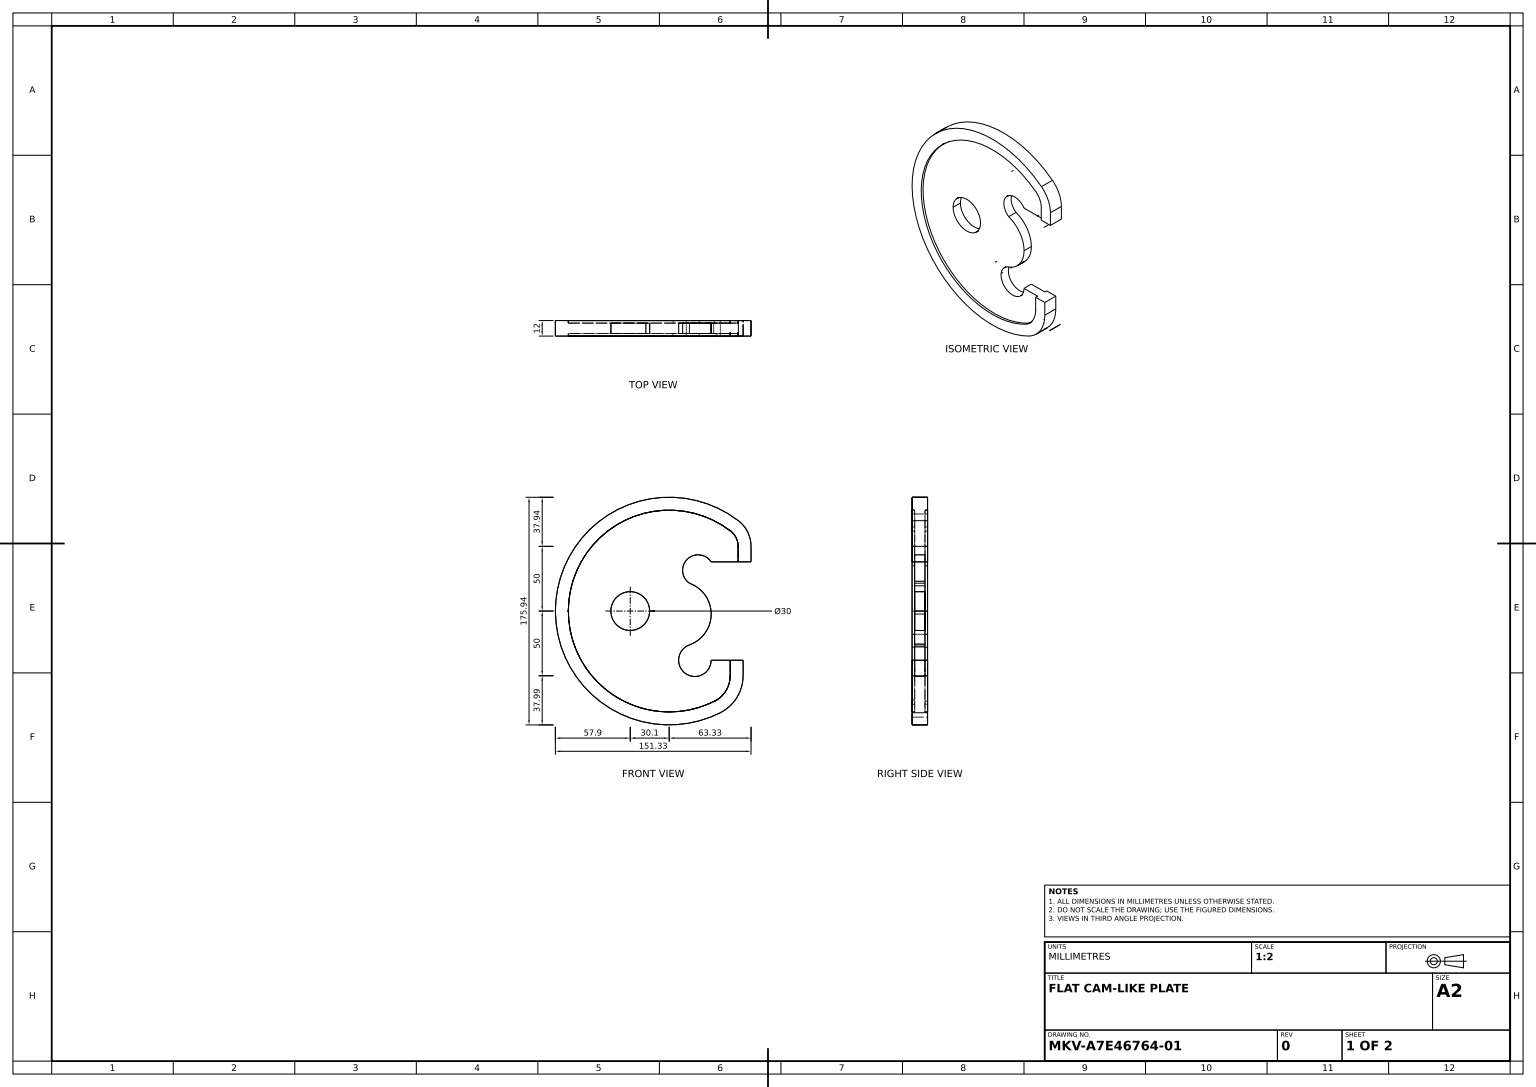
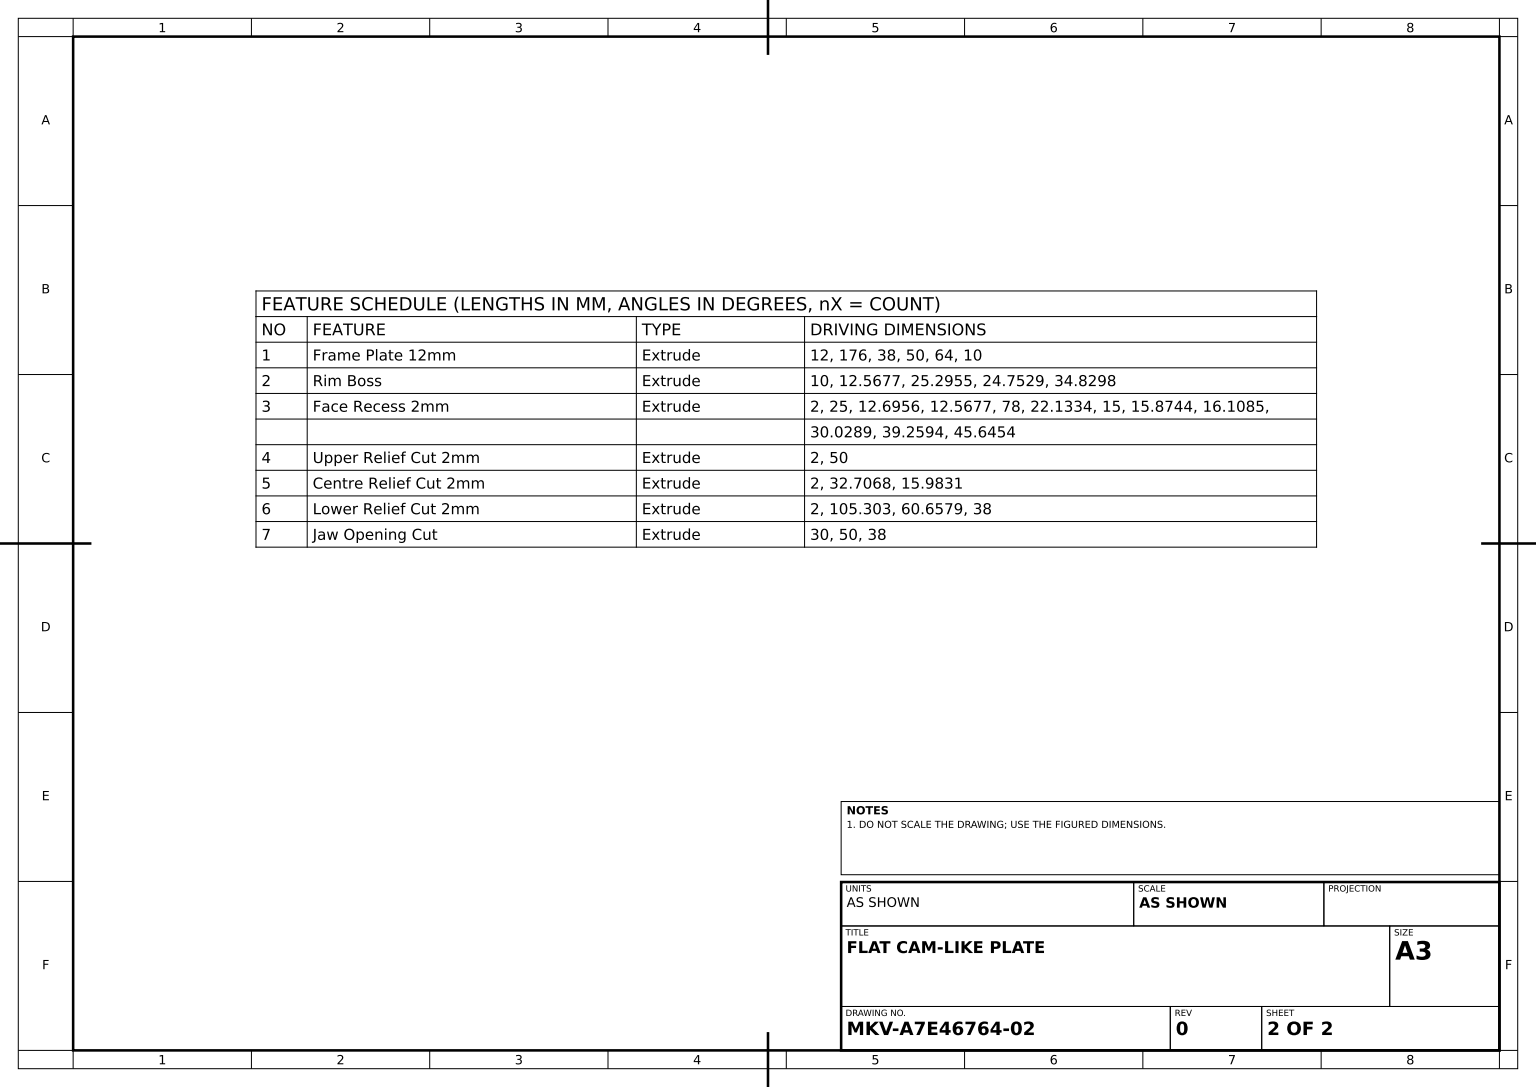
from build123d import *

# Parameters (mm, degrees)
FRAME_PLATE_12MM_DEPTH      = 6
RIM_BOSS_DEPTH              = 10
FACE_RECESS_2MM_DEPTH       = 2
UPPER_START                 = 2
UPPER_RELIEF_CUT_SKETCH_R   = 25
UPPER_RELIEF_CUT_2MM_DEPTH  = 2
CENTRE_RELIEF_CUT_2MM_DEPTH = 2
LOWER_RELIEF_CUT_SKETCH_R   = 52.651518039
LOWER_RELIEF_CUT_2MM_DEPTH  = 2
JAW_OPENING_SKETCH_R        = 15
JAW_OPENING_CUT_DEPTH       = 125.85191228


with BuildPart() as part:
    # Frame Profile Sketch → Frame Plate 12mm (new, symmetric)
    with BuildSketch(Plane.XY):
        with BuildLine():
            Line((57.219040426, -50), (57.219040426, -38))
            Line((57.219040426, -38), (47.219040426, -38))
            Line((47.219040426, -38), (47.219040426, -50))
            ThreePointArc((47.219040426, -50), (43.953561552, -61.533330749), (35.126520593, -69.642857143))
            ThreePointArc((35.126520593, -69.642857143), (-77.659797107, 7.277081367), (47.453139554, 61.904761905))
            ThreePointArc((47.453139554, 61.904761905), (51.779005163, 56.637617931), (53.327535793, 50))
            Line((53.327535793, 50), (53.327535793, 38))
            Line((53.327535793, 38), (63.327535793, 38))
            Line((63.327535793, 38), (63.327535793, 50))
            ThreePointArc((63.327535793, 50), (60.74665141, 61.062696552), (53.536875394, 69.841269841))
            ThreePointArc((53.536875394, 69.841269841), (-87.616181352, 8.210040517), (39.629920669, -78.571428571))
            ThreePointArc((39.629920669, -78.571428571), (52.469252974, -66.775753816), (57.219040426, -50))
        make_face()
    extrude(amount=FRAME_PLATE_12MM_DEPTH, both=True)

    # Rim Boss Sketch → Rim Boss (add)
    with BuildSketch(Plane.XY.offset(6)):
        with BuildLine():
            Line((53.327535793, 38), (32.46615526, 38))
            ThreePointArc((32.46615526, 38), (13.979168764, 40.044097465), (15.696546582, 21.523902608))
            ThreePointArc((15.696546582, 21.523902608), (32.534616457, -2.315840538), (15.696546582, -26.155583684))
            ThreePointArc((15.696546582, -26.155583684), (12.648035491, -48.265354025), (32.46615526, -38))
            Line((32.46615526, -38), (47.219040426, -38))
            Line((47.219040426, -38), (47.219040426, -50))
            ThreePointArc((47.219040426, -50), (43.953561552, -61.533330749), (35.126520593, -69.642857143))
            ThreePointArc((35.126520593, -69.642857143), (-77.659797107, 7.277081367), (47.453139554, 61.904761905))
            ThreePointArc((47.453139554, 61.904761905), (51.779005163, 56.637617931), (53.327535793, 50))
            Line((53.327535793, 50), (53.327535793, 38))
        make_face()
    extrude(amount=-RIM_BOSS_DEPTH)

    # Face Recess Sketch → Face Recess 2mm (cut)
    with BuildSketch(Plane.XY.offset(6)):
        with BuildLine():
            ThreePointArc((36.866729899, -68.73750233), (44.45885626, -60.703554629), (47.219040426, -50))
            Line((47.219040426, -50), (47.219040426, -38))
            Line((47.219040426, -38), (32.46615526, -38))
            ThreePointArc((32.46615526, -38), (30.153940112, -45.264433679), (24.06810264, -49.855829743))
            ThreePointArc((24.06810264, -49.855829743), (7.879587743, -42.091412935), (15.644004551, -25.902898038))
            ThreePointArc((15.644004551, -25.902898038), (32.325529371, -3.417209672), (17.682148152, 20.445959399))
            ThreePointArc((17.682148152, 20.445959399), (16.663921846, 20.938096482), (15.696546582, 21.523902608))
            ThreePointArc((15.696546582, 21.523902608), (13.979168764, 40.044097465), (32.46615526, 38))
            Line((32.46615526, 38), (53.327535793, 38))
            Line((53.327535793, 38), (53.327535793, 50))
            ThreePointArc((53.327535793, 50), (51.779005163, 56.637617931), (47.453139554, 61.904761905))
            ThreePointArc((47.453139554, 61.904761905), (-77.745163176, 6.299968474), (36.866729899, -68.73750233))
        make_face()
    extrude(amount=-FACE_RECESS_2MM_DEPTH, mode=Mode.SUBTRACT)

    # Upper Relief Cut Sketch → Upper Relief Cut 2mm (cut)
    with BuildSketch(Plane.XY.offset(4).offset(UPPER_START)):
        with Locations((7.349665755, -2.318921614)):
            Circle(UPPER_RELIEF_CUT_SKETCH_R)
    extrude(amount=-UPPER_RELIEF_CUT_2MM_DEPTH, mode=Mode.SUBTRACT)

    # Centre Relief Cut Sketch → Centre Relief Cut 2mm (cut)
    with BuildSketch(Plane.XY.offset(4)):
        with BuildLine():
            ThreePointArc((23.833190109, -22.398989717), (-15.184880461, 28.968173855), (4.862308851, -32.34337094))
            ThreePointArc((4.862308851, -32.34337094), (27.276572021, -52.035475846), (23.833190109, -22.398989717))
        make_face()
    extrude(amount=CENTRE_RELIEF_CUT_2MM_DEPTH, mode=Mode.SUBTRACT)

    # Lower Relief Cut Sketch → Lower Relief Cut 2mm (cut)
    with BuildSketch(Plane.XY.offset(4)):
        with Locations((-7.330378767, 0)):
            Circle(LOWER_RELIEF_CUT_SKETCH_R)
    extrude(amount=LOWER_RELIEF_CUT_2MM_DEPTH, mode=Mode.SUBTRACT)

    # Jaw Opening Sketch → Jaw Opening Cut (cut, through all)
    with BuildSketch(Plane.XY.offset(4)):
        with Locations((-30.10151943, 0)):
            Circle(JAW_OPENING_SKETCH_R)
    extrude(amount=-JAW_OPENING_CUT_DEPTH, mode=Mode.SUBTRACT)


solid = part.part
